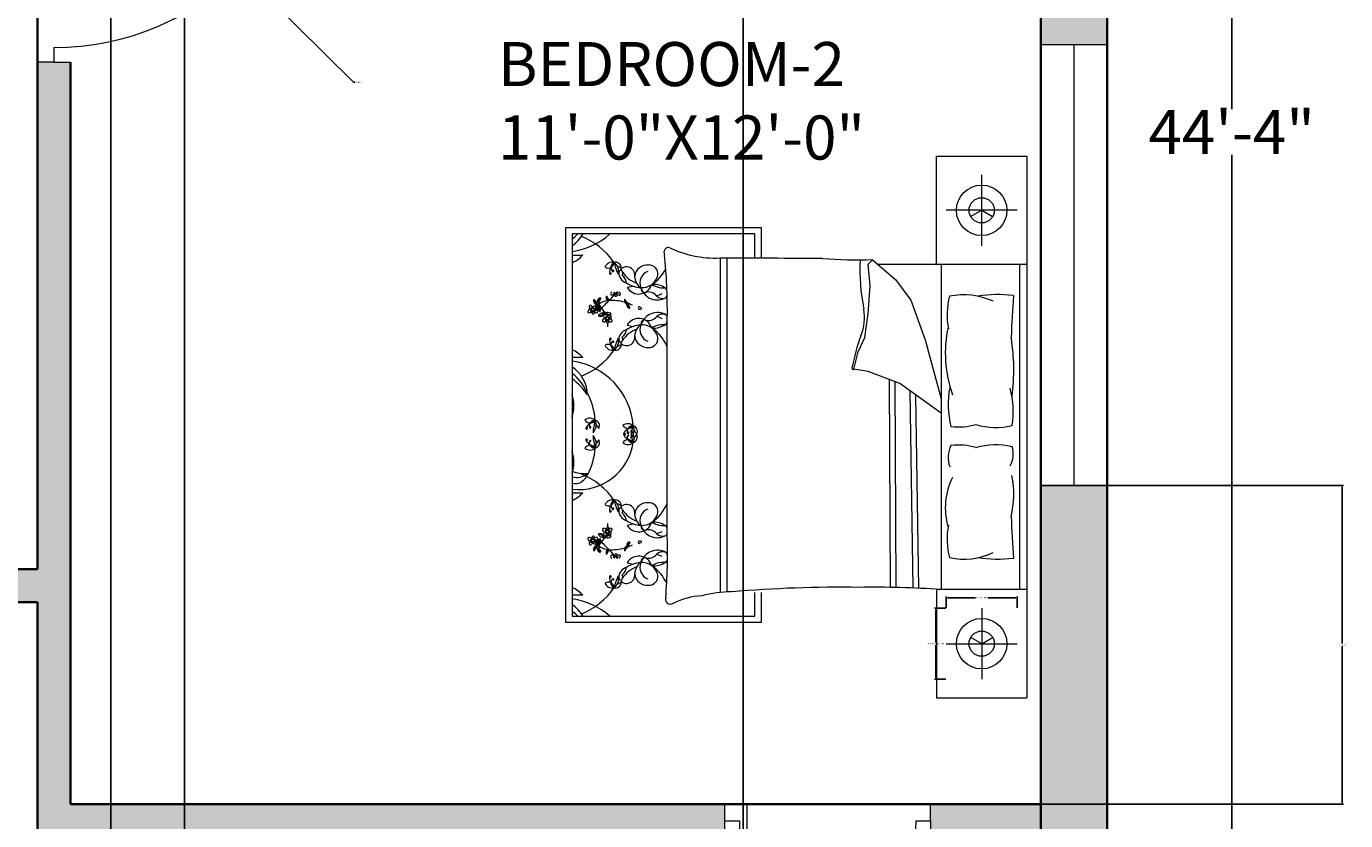
# Model space of a CAD drawing. Units: inches. Extents: x -13 to 349, y -556 to 61.
# Tile 3 of 6: x 170 to 349, y -351 to -243. Entities that reach past the tile are written whole.
import ezdxf

# ---------------------------------------------------------------- set-up
doc = ezdxf.new("R2010")
doc.units = ezdxf.units.IN
doc.header["$MEASUREMENT"] = 0
for name, color, linetype, lineweight in [('A-ANNO-DIMS', 2, 'Continuous', 18), ('A-AREA-IDEN', 7, 'Continuous', 18), ('A-DOOR', 3, 'Continuous', 20), ('A-FURN', 8, 'Continuous', 13), ('A-GLAZ', 5, 'Continuous', 18), ('A-WALL', 7, 'Continuous', 35), ('A-WALL-PATT', 8, 'Continuous', 13)]:
    doc.layers.add(name, color=color, linetype=linetype, lineweight=lineweight)
doc.styles.get("Standard").update_dxf_attribs({"font": 'arial.ttf'})
doc.dimstyles.get("Standard").update_dxf_attribs({"dimtxt": 0.18, "dimasz": 0.18, "dimexe": 0.18, "dimexo": 0.0625, "dimgap": 0.09, "dimtad": 0, "dimtih": 1, "dimtoh": 1, "dimdec": 0, "dimzin": 0, "dimdsep": 46, "dimlunit": 3, "dimtxsty": 'Standard', "dimcen": 0.09, "dimadec": 0, "dimazin": 0, "dimtfac": 1, "dimtdec": 0, "dimtofl": 0, "dimtmove": 0, "dimatfit": 3, "dimfxl": 1, "dimtolj": 1, "dimtzin": 0, "dimarcsym": 0})

# ---------------------------------------------------------------- blocks, each defined once
blk = doc.blocks.new('*D3')
at = {"layer": 'A-ANNO-DIMS', "color": 0, "lineweight": -2, "transparency": 16777216}
for p, q in [((316.82, 8.29), (333.9, 8.29)), ((333.72, 8.11), (333.72, -254.62)), ((333.72, -523.53), (333.72, -260.8)), ((316.82, -523.71), (333.9, -523.71))]:
    blk.add_line(p, q, dxfattribs=at)
at = {"layer": 'A-ANNO-DIMS', "color": 0, "transparency": 16777216}
for points in [[(333.69, 8.11), (333.75, 8.11), (333.72, 8.29)], [(333.69, -523.53), (333.75, -523.53), (333.72, -523.71)]]:
    blk.add_solid(points, dxfattribs=at)
at = {"layer": 'Defpoints', "color": 0, "transparency": 16777216}
for p in [(316.76, 8.29), (316.76, -523.71), (333.72, -523.71)]:
    blk.add_point(p, dxfattribs=at)
at = {"layer": 'A-ANNO-DIMS', "color": 0, "transparency": 16777216, "insert": (333.72, -257.71), "char_height": 6, "attachment_point": 5}
blk.add_mtext('\\A1;44\'-4"', dxfattribs=at)
blk = doc.blocks.new('DOOR-SWING-36IN')
for p, q in [((36, 40), (33.75, 40)), ((36, 38), (36, 40)), ((36, 40), (38.25, 40)), ((38.25, 3), (0, 3)), ((36, 2), (0, 2)), ((36, 0), (36, 2)), ((33.75, 0), (38.25, 0))]:
    blk.add_line(p, q)
blk.add_arc((36, 2), 36, 90, 180)
blk = doc.blocks.new('DOOR-SWING-24IN')
for p, q in [((4.5, 28), (0, 28)), ((2.25, 28), (2.25, 26)), ((2.25, 26), (26.25, 26)), ((0, 25), (26.25, 25)), ((2.25, 2), (2.25, 0)), ((2.25, 0), (0, 0)), ((2.25, 0), (4.5, 0))]:
    blk.add_line(p, q)
blk.add_arc((2.25, 26), 24, 270, 0)
blk = doc.blocks.new('WIN-60IN-D9')
for p, q in [((0, 60), (0, 0)), ((9, 60), (0, 60)), ((4.5, 60), (4.5, 0)), ((9, 0), (9, 60)), ((0, 0), (9, 0))]:
    blk.add_line(p, q)
blk = doc.blocks.new('BEDSIDE-LAMP-SM')
for p, q in [((4.82, 9.64), (4.82, 0)), ((0, 4.82), (9.64, 4.82))]:
    blk.add_line(p, q)
for points in [[(4.82, 4.82), (3.33, 5.68)], [(4.82, 4.82), (6.31, 5.68)]]:
    blk.add_lwpolyline(points)
for radius in [3.44, 1.72]:
    blk.add_circle((4.82, 4.82), radius)
blk = doc.blocks.new('*D32')
at = {"layer": 'A-ANNO-DIMS', "color": 0, "lineweight": -2, "transparency": 16777216}
for p, q in [((294.83, -322.55), (293.27, -322.55)), ((293.45, -322.73), (293.45, -327.19)), ((293.45, -332.01), (293.45, -327.55)), ((294.83, -332.19), (293.27, -332.19))]:
    blk.add_line(p, q, dxfattribs=at)
at = {"layer": 'A-ANNO-DIMS', "color": 0, "transparency": 16777216}
for points in [[(293.42, -322.73), (293.48, -322.73), (293.45, -322.55)], [(293.42, -332.01), (293.48, -332.01), (293.45, -332.19)]]:
    blk.add_solid(points, dxfattribs=at)
at = {"layer": 'Defpoints', "color": 0, "transparency": 16777216}
for p in [(293.45, -322.55), (294.89, -322.55), (294.89, -332.19)]:
    blk.add_point(p, dxfattribs=at)
at = {"layer": 'A-ANNO-DIMS', "color": 0, "transparency": 16777216, "insert": (293.45, -327.37), "char_height": 0.18, "attachment_point": 5}
blk.add_mtext('\\A1;LAMP B 0\'-9 1/2" TYP.', dxfattribs=at)
blk = doc.blocks.new('*D33')
at = {"layer": 'A-ANNO-DIMS', "color": 0, "lineweight": -2, "transparency": 16777216}
for p, q in [((294.89, -322.49), (294.89, -320.93)), ((295.07, -321.11), (298.86, -321.11)), ((304.35, -321.11), (300.56, -321.11)), ((304.53, -322.49), (304.53, -320.93))]:
    blk.add_line(p, q, dxfattribs=at)
at = {"layer": 'A-ANNO-DIMS', "color": 0, "transparency": 16777216}
for points in [[(295.07, -321.08), (295.07, -321.14), (294.89, -321.11)], [(304.35, -321.08), (304.35, -321.14), (304.53, -321.11)]]:
    blk.add_solid(points, dxfattribs=at)
at = {"layer": 'Defpoints', "color": 0, "transparency": 16777216}
for p in [(304.53, -321.11), (294.89, -322.55), (304.53, -322.55)]:
    blk.add_point(p, dxfattribs=at)
at = {"layer": 'A-ANNO-DIMS', "color": 0, "transparency": 16777216, "insert": (299.71, -321.11), "char_height": 0.18, "attachment_point": 5}
blk.add_mtext('\\A1;0\'-9 1/2" TYP.', dxfattribs=at)
blk = doc.blocks.new('*D34')
at = {"layer": 'A-ANNO-DIMS', "color": 0, "lineweight": -2, "transparency": 16777216}
for p, q in [((267.26, -200.78), (267.26, -555.89)), ((307.76, -200.78), (307.76, -555.89)), ((267.44, -555.71), (286.97, -555.71)), ((307.58, -555.71), (288.04, -555.71))]:
    blk.add_line(p, q, dxfattribs=at)
at = {"layer": 'A-ANNO-DIMS', "color": 0, "transparency": 16777216}
for points in [[(267.44, -555.68), (267.44, -555.74), (267.26, -555.71)], [(307.58, -555.68), (307.58, -555.74), (307.76, -555.71)]]:
    blk.add_solid(points, dxfattribs=at)
at = {"layer": 'Defpoints', "color": 0, "transparency": 16777216}
for p in [(267.26, -200.71), (307.76, -200.71), (307.76, -555.71)]:
    blk.add_point(p, dxfattribs=at)
at = {"layer": 'A-ANNO-DIMS', "color": 0, "transparency": 16777216, "insert": (287.51, -555.71), "char_height": 0.18, "attachment_point": 5}
blk.add_mtext('\\A1;3\'-4 1/2"', dxfattribs=at)
blk = doc.blocks.new('*D37')
at = {"layer": 'A-ANNO-DIMS', "color": 0, "lineweight": -2, "transparency": 16777216}
for p, q in [((181.26, -353.65), (181.26, 40.47)), ((181.44, 40.29), (185.86, 40.29)), ((191.08, 40.29), (186.65, 40.29)), ((191.26, -353.65), (191.26, 40.47))]:
    blk.add_line(p, q, dxfattribs=at)
at = {"layer": 'A-ANNO-DIMS', "color": 0, "transparency": 16777216}
for points in [[(181.44, 40.32), (181.44, 40.26), (181.26, 40.29)], [(191.08, 40.32), (191.08, 40.26), (191.26, 40.29)]]:
    blk.add_solid(points, dxfattribs=at)
at = {"layer": 'Defpoints', "color": 0, "transparency": 16777216}
for p in [(191.26, 40.29), (181.26, -353.71), (191.26, -353.71)]:
    blk.add_point(p, dxfattribs=at)
at = {"layer": 'A-ANNO-DIMS', "color": 0, "transparency": 16777216, "insert": (186.26, 40.29), "char_height": 0.18, "attachment_point": 5}
blk.add_mtext('\\A1;0\'-10"', dxfattribs=at)
blk = doc.blocks.new('*D42')
at = {"layer": 'A-ANNO-DIMS', "color": 0, "lineweight": -2, "transparency": 16777216}
for p, q in [((307.82, -305.84), (348.94, -305.84)), ((348.76, -306.02), (348.76, -327.34)), ((348.76, -349.03), (348.76, -327.71)), ((307.82, -349.21), (348.94, -349.21))]:
    blk.add_line(p, q, dxfattribs=at)
at = {"layer": 'A-ANNO-DIMS', "color": 0, "transparency": 16777216}
for points in [[(348.73, -306.02), (348.79, -306.02), (348.76, -305.84)], [(348.73, -349.03), (348.79, -349.03), (348.76, -349.21)]]:
    blk.add_solid(points, dxfattribs=at)
at = {"layer": 'Defpoints', "color": 0, "transparency": 16777216}
for p in [(307.76, -305.84), (307.76, -349.21), (348.76, -349.21)]:
    blk.add_point(p, dxfattribs=at)
at = {"layer": 'A-ANNO-DIMS', "color": 0, "transparency": 16777216, "insert": (348.76, -327.53), "char_height": 0.18, "attachment_point": 5}
blk.add_mtext('\\A1;3\'-7 1/2"', dxfattribs=at)
blk = doc.blocks.new('*D48')
at = {"layer": 'A-ANNO-DIMS', "color": 0, "lineweight": -2, "transparency": 16777216}
for p, q in [((173.42, -210.21), (173.6, -210.21)), ((173.51, -210.3), (173.51, -210.12)), ((214.24, -250.94), (199.09, -235.8)), ((214.42, -250.94), (214.24, -250.94))]:
    blk.add_line(p, q, dxfattribs=at)
at = {"layer": 'A-ANNO-DIMS', "color": 0, "transparency": 16777216}
blk.add_solid([(199.11, -235.77), (199.07, -235.82), (198.96, -235.67)], dxfattribs=at)
at = {"layer": 'Defpoints', "color": 0, "transparency": 16777216}
for p in [(173.51, -210.21), (198.96, -235.67)]:
    blk.add_point(p, dxfattribs=at)
at = {"layer": 'A-ANNO-DIMS', "color": 0, "transparency": 16777216, "insert": (215.03, -250.94), "char_height": 0.18, "attachment_point": 5}
blk.add_mtext('\\A1;4X R3\'-0"', dxfattribs=at)

msp = doc.modelspace()

# ---------------------------------------------------------------- hatches: boundary and pattern name
at = {"layer": 'A-WALL-PATT'}
h = msp.add_hatch(color=256, dxfattribs=at)
h.dxf.hatch_style = 1
h.paths.add_polyline_path([(316.76, 8.29), (171.26, 8.29), (171.26, -0.71), (307.76, -0.71), (307.76, -52.19), (316.76, -52.19)])
h.paths.add_polyline_path([(175.76, -0.71), (171.26, -0.71), (171.26, -82.21), (165.24, -82.21), (165.24, -86.71), (171.26, -86.71), (171.26, -101.71), (173.51, -101.71), (175.76, -101.71)])
h.paths.add_polyline_path([(171.26, -25.21), (165.17, -25.21), (165.17, -34.21), (171.26, -34.21)])
h.paths.add_polyline_path([(141.17, -25.21), (127.76, -25.21), (127.76, -34.21), (141.17, -34.21)])
h.paths.add_polyline_path([(28.76, -25.21), (24.26, -25.21), (19.76, -25.21), (19.76, -78.88), (28.76, -78.88)])
h.paths.add_polyline_path([(99.76, -29.71), (99.76, -25.21), (28.76, -25.21), (28.76, -34.21), (99.76, -34.21)])
h.paths.add_polyline_path([(135.26, -86.71), (143.68, -86.71), (143.68, -82.21), (135.26, -82.21), (135.26, -34.21), (130.76, -34.21), (130.76, -101.71), (133.01, -101.71), (135.26, -101.71)])
h.paths.add_polyline_path([(135.26, -141.71), (130.76, -141.71), (130.76, -144.71), (28.76, -144.71), (28.76, -149.21), (135.26, -149.21)])
h.paths.add_polyline_path([(28.76, -138.88), (19.76, -138.88), (19.76, -156.62), (28.76, -156.62)])
h.paths.add_polyline_path([(28.76, -192.62), (19.76, -192.62), (19.76, -271.06), (28.76, -271.06)])
h.paths.add_polyline_path([(28.76, -307.06), (19.76, -307.06), (19.76, -385.56), (28.76, -385.56)])
h.paths.add_polyline_path([(28.76, -445.56), (19.76, -445.56), (19.76, -523.71), (28.76, -523.71)])
h.paths.add_polyline_path([(307.76, -431.71), (261.76, -431.71), (261.76, -353.71), (264.76, -353.71), (264.76, -349.21), (175.76, -349.21), (175.76, -248.21), (173.51, -248.21), (171.26, -248.21), (171.26, -317.21), (168.26, -317.21), (168.26, -321.71), (171.26, -321.71), (171.26, -353.71), (257.26, -353.71), (257.26, -431.71), (171.26, -431.71), (171.26, -436.21), (307.76, -436.21)])
h.paths.add_polyline_path([(316.76, -424.85), (307.76, -424.85), (307.76, -436.21), (316.76, -436.21)])
h.paths.add_polyline_path([(316.76, -305.84), (307.76, -305.84), (307.76, -400.85), (316.76, -400.85)])
h.paths.add_polyline_path([(307.76, -349.21), (292.76, -349.21), (292.76, -351.46), (292.76, -353.71), (307.76, -353.71)], flags=17)
h.paths.add_polyline_path([(271.19, -200.71), (267.26, -200.71), (267.26, -186.96), (262.76, -186.96), (262.76, -200.71), (175.76, -200.71), (175.76, -180.21), (173.51, -180.21), (171.26, -180.21), (171.26, -208.21), (175.76, -208.21), (175.76, -205.21), (271.19, -205.21)])
h.paths.add_polyline_path([(316.76, -112.19), (307.76, -112.19), (307.76, -245.84), (316.76, -245.84)])
h.paths.add_polyline_path([(271.33, -144.71), (175.76, -144.71), (175.76, -141.71), (171.26, -141.71), (171.26, -152.21), (175.76, -152.21), (175.76, -149.21), (262.76, -149.21), (262.76, -162.96), (267.26, -162.96), (267.26, -149.21), (271.33, -149.21)])
h.paths.add_polyline_path([(307.76, -200.71), (307.19, -200.71), (307.19, -205.21), (307.76, -205.21)])
h.paths.add_polyline_path([(307.76, -144.71), (307.33, -144.71), (307.33, -149.21), (307.76, -149.21)])

# ---------------------------------------------------------------- linework, layer by layer
at = {"layer": 'A-FURN'}
for p, q in [((305.85, -261), (305.85, -334.74)), ((243.14, -270.73), (269.7, -270.73)), ((243.14, -324.5), (243.14, -270.73)), ((269.7, -270.73), (269.7, -274.9)), ((243.99, -271.59), (243.99, -323.64)), ((268.85, -271.59), (243.99, -271.59)), ((268.85, -274.9), (268.85, -271.59)), ((264.19, -320.4), (264.19, -274.9)), ((265.1, -320.33), (265.1, -274.9)), ((284.25, -275.68), (284.84, -275.09)), ((284.55, -278.67), (284.25, -275.68)), ((284.84, -275.09), (287.98, -277.78)), ((305.85, -275.75), (285.61, -275.75)), ((294.2, -275.75), (294.2, -320)), ((304.91, -320), (304.91, -275.75)), ((287.98, -277.78), (290.07, -280.61)), ((251.47, -278.85), (252.3, -278.69)), ((284.25, -282.41), (284.55, -278.67)), ((290.07, -280.61), (292.01, -285.99)), ((256.94, -312.84), (256.94, -282.9)), ((283.8, -285.69), (284.25, -282.41)), ((251.47, -284.01), (252.3, -284.17)), ((282.9, -287.63), (283.8, -285.69)), ((292.01, -285.99), (294.2, -294.03)), ((282.31, -290.02), (282.9, -287.63)), ((284.25, -290.32), (282.31, -290.02)), ((288.58, -291.97), (284.25, -290.32)), ((287.3, -319.73), (287.19, -291.44)), ((288.06, -319.73), (287.95, -291.73)), ((294.2, -296.01), (288.58, -291.97)), ((290.38, -319.77), (290, -292.99)), ((291.14, -319.8), (290.77, -293.54)), ((251.47, -311.22), (252.3, -311.06)), ((251.47, -316.37), (252.3, -316.54)), ((268.85, -323.64), (268.85, -320.39)), ((269.7, -320.41), (269.7, -324.5)), ((269.7, -324.5), (243.14, -324.5)), ((243.99, -323.64), (268.85, -323.64))]:
    msp.add_line(p, q, dxfattribs=at)
for points in [[(293.56, -275.75), (293.56, -261), (305.85, -261)], [(305.85, -320), (293.56, -320), (293.56, -334.74), (305.85, -334.74)]]:
    msp.add_lwpolyline(points, dxfattribs=at)
for points in [[(278.09, -274.93, 0.001242), (264.1, -274.9, -0.127202), (257.13, -273.42)], [(304.02, -279.98, 0.074897), (299.2, -280.07, -0.472817)], [(298.93, -297.53, 0.14099), (303.84, -297.67, 0.235245)], [(298.93, -300.67, -0.14099), (303.84, -300.53, -0.235245)], [(304.02, -315.76, -0.074897), (299.2, -315.67, 0.472817)], [(265.69, -320.31, 0.056112), (261.63, -320.84, 0.095341), (257.72, -321.88)]]:
    msp.add_lwpolyline(points, format="xyb", dxfattribs=at)
for centre in [(246.82, -281.89), (248.8, -283.11), (248.8, -312.11), (246.82, -313.34)]:
    msp.add_circle(centre, 0.188, dxfattribs=at)
for centre, radius, start, end in [((240.53, -267.56), 5.85, 306.3036, 316.4814), ((241.41, -269.25), 4.69, 303.4617, 330.1116), ((242.7, -264.42), 9.63, 277.745, 311.8856), ((241.74, -280.89), 9.63, 34.3865, 68.5908), ((242.49, -271.88), 3.92, 292.5547, 318.9546), ((244.6, -261.15), 13.32, 267.4081, 273.6519), ((257.17, -274.1), 0.68, 93.98, 207.3412), ((180.18, -282.02), 76.77, 359.3433, 5.6887), ((249.46, -276.5), 1.07, 77.7115, 159.0387), ((248.89, -275.43), 0.804, 238.4633, 358.2869), ((251.52, -277.06), 2.44, 138.8402, 177.9352), ((250.06, -276.15), 0.788, 117.6827, 223.7762), ((249.88, -276.23), 0.798, 2.9516, 103.728), ((256.27, -273.99), 6.74, 192.5173, 207.1824), ((248.8, -276.69), 1.52, 345.4653, 54.2343), ((251.1, -274.6), 1.64, 211.3827, 255.2969), ((251.41, -277.17), 1.11, 350.264, 160.8688), ((254.25, -277.57), 1.76, 84.9449, 172.8857), ((254.43, -277.06), 1.25, 354.4856, 91.0538), ((251.75, -273.81), 5.58, 303.6671, 333.2997), ((283.01, -207.47), 67.64, 265.8294, 271.553), ((310.96, -276.35), 27.83, 177.4519, 191.3392), ((249.21, -276.97), 0.12, 177.9352, 11.4834), ((249.27, -276.96), 0.0581, 11.4834, 127.9409), ((249.56, -276.62), 0.104, 223.7762, 159.7183), ((251.74, -276.9), 1.38, 175.969, 254.3045), ((250.21, -276.94), 0.678, 333.9755, 53.2681), ((249.91, -278.39), 1.47, 6.1662, 51.5825), ((253.85, -274.97), 3.48, 211.2614, 251.7045), ((254.64, -277.27), 2.14, 182.3591, 234.0401), ((254.92, -278.27), 1.71, 111.5819, 201.4221), ((253.51, -276.68), 2.22, 265.2933, 346.921), ((244.23, -275.55), 7, 313.1541, 322.0459), ((249.38, -279.76), 0.144, 142.4737, 265.053), ((249.57, -279.73), 0.31, 127.7621, 169.0403), ((249.4, -279.47), 0.436, 265.053, 338.3618), ((249.98, -280.06), 0.57, 113.4276, 137.6104), ((249.91, -279.47), 0.188, 183.2768, 356.7232), ((250.05, -279.81), 0.307, 139.7889, 227.6792), ((249.95, -279.92), 0.162, 227.6792, 350.3487), ((249.33, -279.81), 0.615, 353.0852, 15.7171), ((249.73, -279.88), 0.388, 350.3487, 43.6538), ((250.45, -279.48), 0.452, 198.7263, 262.5032), ((250.09, -279.69), 0.179, 1.1081, 91.8675), ((250.2, -279.73), 0.313, 11.5637, 52.6358), ((250.43, -279.79), 0.145, 255.2356, 54.9248), ((253.57, -274.94), 3.96, 236.2883, 266.5076), ((253.06, -277.94), 1.83, 209.9085, 343.1337), ((253.83, -279.1), 0.458, 167.3041, 285.1471), ((255.07, -281.29), 2.84, 122.7011, 126.3445), ((255.6, -278.22), 2.35, 199.2822, 299.1751), ((254.34, -281), 1.51, 41.5653, 105.1471), ((256.4, -275.86), 3.06, 238.8218, 279.1554), ((255.07, -281.29), 2.84, 55.785, 94.7304), ((255.18, -277.87), 2.12, 277.436, 299.9149), ((256.13, -279.64), 0.888, 30.0293, 52.325), ((297.27, -289.38), 9.5, 65.1316, 101.7583), ((246.67, -281.5), 0.371, 157.4086, 261.4386), ((246.47, -281.49), 0.186, 58.0499, 135.6268), ((246.66, -281.61), 0.124, 172.906, 277.132), ((246.25, -281.84), 0.592, 14.7558, 58.0499), ((247.08, -281.68), 0.256, 36.1046, 181.4281), ((247.09, -280.67), 0.21, 124.3538, 214.3923), ((247.4, -280.71), 0.489, 190.3057, 287.1958), ((246.93, -281.48), 0.259, 270.0645, 331.1507), ((247.15, -281.54), 0.295, 221.8413, 265.7877), ((247.54, -280.53), 0.568, 176.9701, 248.2913), ((251.59, -277.54), 5.49, 212.6784, 216.3746), ((247.15, -281.65), 0.184, 263.7526, 41.7054), ((247.35, -280.66), 0.217, 216.3746, 291.7548), ((249.27, -283.71), 3.06, 124.0033, 132.4917), ((246.12, -284.1), 3.27, 63.7819, 68.2913), ((247.87, -281.58), 0.52, 128.3208, 208.8162), ((247.87, -280.82), 0.489, 122.8155, 187.3992), ((247.49, -281.02), 0.164, 289.3605, 111.7548), ((247.61, -281.02), 0.164, 221.8703, 44.2646), ((248.36, -281.49), 0.856, 157.2305, 229.0635), ((248.08, -280.88), 0.568, 109.4799, 177.6828), ((248.07, -281.21), 0.504, 174.4544, 220.6188), ((245.2, -284.03), 3.67, 30.544, 49.818), ((247.78, -280.52), 0.21, 56.8636, 146.9021), ((247.89, -280.75), 0.217, 148.8844, 224.2646), ((247.23, -281.93), 0.606, 340.0041, 40.6188), ((252.4, -283.48), 5.49, 145.1882, 148.8844), ((249.27, -283.71), 3.06, 94.756, 119.2041), ((255.79, -288.12), 10.08, 132.2412, 142.1744), ((250.7, -280.1), 2.08, 178.3264, 187.1302), ((248.46, -280.39), 0.387, 11.3256, 64.4621), ((249.77, -279.83), 1.17, 190.2588, 210.656), ((248.99, -280.31), 0.354, 188.3432, 274.2869), ((249.3, -280.11), 0.618, 210.656, 242.6341), ((249.77, -279.58), 1.18, 218.2101, 226.3071), ((248.89, -280.58), 0.15, 325.7657, 67.4417), ((249.42, -286.75), 6.11, 73.5842, 93.8277), ((253.18, -280.54), 2.08, 178.3264, 187.1302), ((250.94, -280.83), 0.387, 11.3256, 64.4621), ((252.25, -280.27), 1.17, 190.2588, 210.656), ((251.47, -280.75), 0.354, 188.3432, 274.2869), ((251.78, -280.55), 0.618, 210.656, 242.6341), ((252.25, -280.02), 1.18, 218.2101, 226.3071), ((251.37, -281.01), 0.15, 325.7657, 67.4417), ((251.8, -281.29), 0.354, 147.5332, 233.4768), ((252.12, -281.11), 0.618, 179.1859, 211.164), ((251.51, -281.25), 0.15, 354.3784, 96.0543), ((249.42, -286.75), 6.11, 63.0032, 69.8941), ((252.58, -280.82), 1.17, 211.164, 231.5612), ((252.79, -279.88), 2.08, 234.6898, 243.4936), ((252.8, -280.95), 1.18, 195.5129, 203.6099), ((251.47, -281.72), 0.387, 357.3579, 50.4944), ((253.14, -281.64), 0.142, 12.7051, 190.4384), ((253.22, -281.63), 0.231, 190.4384, 10.4136), ((256.3, -279.27), 1.1, 221.5653, 293.8354), ((256.13, -279.64), 0.888, 314.4517, 333.558), ((304.88, -282.61), 9.88, 165.1039, 191.0369), ((1005.83, -320.63), 702.99, 176.68521, 177.14978), ((246.28, -282.17), 0.144, 142.4737, 265.053), ((246.47, -282.14), 0.31, 61.2196, 169.0403), ((246.31, -281.88), 0.436, 265.053, 338.3618), ((246.88, -282.48), 0.57, 113.4276, 137.6104), ((246.96, -282.23), 0.307, 139.7889, 227.6792), ((246.86, -282.33), 0.162, 227.6792, 350.3487), ((246.23, -282.22), 0.615, 353.0852, 15.7171), ((246.64, -282.3), 0.388, 350.3487, 43.6538), ((247.35, -281.89), 0.452, 198.7263, 262.5032), ((247, -282.1), 0.179, 1.1081, 91.8675), ((247.11, -282.15), 0.313, 11.5637, 86.365), ((247.33, -282.2), 0.145, 255.2356, 54.9248), ((247.96, -281.54), 0.622, 207.7043, 254.3516), ((247.56, -281.9), 0.856, 270.278, 342.111), ((248.13, -282.97), 0.606, 98.7227, 159.3375), ((247.82, -282.19), 0.622, 244.9899, 291.6373), ((247.96, -281.87), 0.504, 278.7227, 324.8872), ((247.87, -282.28), 0.52, 290.5253, 358.5375), ((248.26, -283.4), 0.144, 142.4737, 265.053), ((248.45, -283.37), 0.31, 61.2196, 169.0403), ((248.29, -283.11), 0.436, 265.053, 338.3618), ((248.65, -282.73), 0.371, 157.4086, 261.4386), ((248.45, -282.72), 0.186, 58.0499, 135.6268), ((248.89, -282.13), 0.52, 182.8499, 266.1226), ((248.68, -281.77), 0.504, 231.7607, 277.9252), ((249.08, -281.68), 0.856, 214.5369, 286.3699), ((248.86, -283.7), 0.57, 113.4276, 137.6104), ((248.64, -282.84), 0.124, 172.906, 277.132), ((248.23, -283.06), 0.592, 14.7558, 58.0499), ((245.2, -284.03), 3.67, 23.0501, 23.8477), ((248.94, -283.45), 0.307, 139.7889, 227.6792), ((248.84, -282.87), 0.606, 37.3105, 97.9252), ((249.06, -282.91), 0.256, 36.1046, 181.4281), ((248.21, -283.45), 0.615, 353.0852, 15.7171), ((248.9, -282.03), 0.622, 265.0106, 311.658), ((248.61, -283.52), 0.388, 350.3487, 43.6538), ((248.91, -282.71), 0.259, 270.0645, 331.1507), ((249.13, -282.77), 0.295, 221.8413, 265.7877), ((249.33, -283.12), 0.452, 198.7263, 262.5032), ((248.98, -283.33), 0.179, 1.1081, 91.8675), ((249.13, -282.88), 0.184, 263.7526, 41.7054), ((249.09, -283.37), 0.313, 11.5637, 86.365), ((249.31, -283.43), 0.145, 255.2356, 54.9248), ((253.06, -284.92), 1.83, 16.8663, 150.0915), ((253.83, -283.76), 0.458, 74.8529, 192.6959), ((255.6, -284.64), 2.35, 60.8249, 160.7178), ((254.34, -281.86), 1.51, 254.8529, 318.4347), ((255.18, -284.99), 2.12, 60.0851, 82.564), ((256.3, -283.6), 1.1, 66.1646, 138.4347), ((256.13, -283.22), 0.888, 23.229, 45.5483), ((277.78, -283), 6, 336.2616, 11.3392), ((248.84, -283.56), 0.162, 227.6792, 350.3487), ((245.2, -284.03), 3.67, 357.1071, 4.7585), ((251.74, -285.96), 1.38, 105.6955, 184.031), ((249.91, -284.47), 1.47, 308.4175, 353.8338), ((253.85, -287.89), 3.48, 108.2955, 148.7386), ((253.57, -287.92), 3.96, 93.4924, 123.7117), ((254.64, -285.6), 2.14, 125.9599, 177.6409), ((254.92, -284.6), 1.71, 158.5779, 248.4181), ((253.51, -286.18), 2.22, 13.079, 94.7067), ((255.07, -281.57), 2.84, 233.6555, 237.2989), ((256.4, -287), 3.06, 79.7133, 121.1782), ((255.07, -281.57), 2.84, 265.2696, 304.215), ((251.75, -289.05), 5.58, 21.4941, 56.3329), ((256.13, -283.22), 0.888, 307.675, 336.7144), ((311.9, -287.82), 17.14, 168.0397, 199.2615), ((248.89, -287.43), 0.804, 1.7131, 121.5367), ((249.46, -286.36), 1.07, 200.9613, 282.2885), ((249.21, -285.89), 0.12, 348.5166, 182.0648), ((251.52, -285.8), 2.44, 182.0648, 221.1598), ((249.27, -285.9), 0.0581, 232.0591, 348.5166), ((250.06, -286.71), 0.788, 136.2238, 242.3173), ((249.6, -286.25), 0.0628, 200.2667, 136.2271), ((248.8, -286.17), 1.52, 305.7657, 14.5347), ((256.27, -288.87), 6.74, 152.8176, 167.4827), ((249.88, -286.63), 0.798, 256.272, 357.0484), ((251.1, -288.26), 1.64, 104.7031, 148.6173), ((251.41, -285.69), 1.11, 199.1312, 9.736), ((250.21, -285.92), 0.678, 306.7319, 26.0245), ((254.25, -285.29), 1.76, 187.1143, 275.0551), ((254.43, -285.8), 1.25, 268.9462, 5.5144), ((310.17, -295.14), 28.6, 160.1194, 169.3383), ((277.33, -290.09), 26.75, 352.2196, 9.497), ((242.49, -290.99), 3.92, 41.0454, 67.4453), ((244.6, -301.71), 13.32, 86.3481, 92.5919), ((242.7, -298.44), 9.63, 4.4623, 82.255), ((241.74, -281.97), 9.63, 291.4092, 325.6135), ((241.41, -293.61), 4.69, 1.272, 56.5383), ((240.53, -295.3), 5.85, 17.8504, 53.6964), ((282.25, -289.86), 0.178, 178.8623, 289.7536), ((238.89, -298.37), 8.7, 34.0123, 54.053), ((308.16, -294.76), 13, 169.8617, 193.6238), ((238.93, -295.01), 5.3, 343.5431, 17.0202), ((237.54, -297.71), 9.63, 4.4623, 27.4146), ((290.85, -295.74), 13.14, 351.5249, 13.96), ((236.2, -297.11), 7.83, 4.3787, 5.6357), ((230.84, -301.24), 13.99, 19.7217, 19.9028), ((246.42, -297.75), 1.07, 47.7873, 129.1145), ((246.45, -296.54), 0.804, 208.5391, 328.3627), ((247.93, -299.26), 2.44, 108.9159, 148.011), ((247.11, -297.75), 0.788, 87.7585, 193.852), ((246.44, -297.91), 0.104, 193.852, 129.9245), ((253.57, -298.97), 6.74, 162.593, 177.2582), ((245.75, -297.58), 1.52, 315.5411, 24.3101), ((248.78, -296.92), 1.64, 181.4585, 225.3727), ((246.92, -297.72), 0.798, 333.0274, 73.8037), ((251.58, -298.49), 1.07, 47.7873, 129.1145), ((251.61, -297.27), 0.804, 208.5391, 328.3627), ((253.09, -300), 2.44, 108.9159, 148.011), ((252.27, -298.48), 0.788, 87.7585, 193.852), ((250.91, -298.32), 1.52, 315.5411, 24.3101), ((258.73, -299.71), 6.74, 162.593, 177.2582), ((252.07, -298.46), 0.798, 333.0274, 73.8037), ((253.94, -297.65), 1.64, 181.4585, 225.3727), ((296.47, -288.83), 9.04, 264.0129, 285.8293), ((245.96, -298.04), 0.12, 148.011, 341.5592), ((245.96, -299.65), 0.12, 18.4408, 211.989), ((246.02, -298.05), 0.0581, 341.5592, 98.0167), ((246.02, -299.63), 0.0581, 261.9833, 18.4408), ((253.57, -298.71), 6.74, 182.7418, 197.407), ((245.75, -300.1), 1.52, 335.6899, 44.4589), ((248.78, -300.77), 1.64, 134.6273, 178.5415), ((246.92, -299.96), 0.798, 286.1963, 26.9726), ((251.61, -300.41), 0.804, 31.6373, 151.4609), ((251.12, -298.77), 0.12, 148.011, 341.5592), ((251.12, -298.91), 0.12, 18.4408, 211.989), ((253.09, -297.69), 2.44, 211.989, 251.0841), ((251.18, -298.79), 0.0581, 341.5592, 98.0167), ((251.18, -298.89), 0.0581, 261.9833, 18.4408), ((252.27, -299.2), 0.788, 166.148, 272.2415), ((251.6, -298.65), 0.104, 193.852, 129.9245), ((251.64, -299.03), 0.0628, 230.1909, 166.0209), ((250.91, -299.36), 1.52, 335.6899, 44.4589), ((258.73, -297.98), 6.74, 182.7418, 197.407), ((252.07, -299.22), 0.798, 286.1963, 26.9726), ((253.94, -300.03), 1.64, 134.6273, 178.5415), ((244.92, -298.93), 7.45, 262.8636, 351.8197), ((238.93, -302.67), 5.3, 342.9798, 16.4569), ((236.2, -300.57), 7.83, 354.3643, 355.6213), ((230.84, -296.45), 13.99, 340.0972, 340.2783), ((246.45, -301.15), 0.804, 31.6373, 151.4609), ((246.42, -299.94), 1.07, 230.8855, 312.2127), ((247.93, -298.42), 2.44, 211.989, 251.0841), ((237.54, -299.98), 9.63, 332.5854, 355.5377), ((247.11, -299.94), 0.788, 166.148, 272.2415), ((246.48, -299.77), 0.0628, 230.1909, 166.0209), ((251.58, -299.2), 1.07, 230.8855, 312.2127), ((299.07, -302.03), 3.91, 155.0183, 198.5407), ((296.47, -309.37), 9.04, 74.1707, 95.9871), ((300.34, -301.54), 3.65, 333.3437, 16.1026), ((245.6, -299.89), 4.31, 248.117, 276.6195), ((244.4, -303.85), 1.73, 256.3898, 349.0739), ((244.64, -302.55), 2.19, 252.8609, 311.9049), ((241.74, -313.26), 9.63, 34.3865, 68.5908), ((304.15, -308.86), 9.39, 153.8761, 196.1746), ((291.11, -307.01), 12.96, 346.3427, 11.1841), ((244.6, -293.52), 13.32, 267.4081, 273.6519), ((242.49, -304.24), 3.92, 292.5547, 318.9546), ((249.46, -308.86), 1.07, 77.7115, 159.0387), ((248.89, -307.8), 0.804, 238.4633, 358.2869), ((251.52, -309.42), 2.44, 138.8402, 177.9352), ((250.06, -308.52), 0.788, 117.6827, 223.7762), ((249.88, -308.6), 0.798, 2.9516, 103.728), ((251.1, -306.96), 1.64, 211.3827, 255.2969), ((248.8, -309.06), 1.52, 345.4653, 54.2343), ((256.27, -306.36), 6.74, 192.5173, 207.1824), ((251.41, -309.53), 1.11, 350.264, 160.8688), ((254.25, -309.94), 1.76, 84.9449, 172.8857), ((254.43, -309.43), 1.25, 354.4856, 91.0538), ((251.75, -306.18), 5.58, 303.6671, 338.5059), ((249.21, -309.34), 0.12, 177.9352, 11.4834), ((249.27, -309.33), 0.0581, 11.4834, 127.9409), ((249.56, -308.99), 0.104, 223.7762, 159.7183), ((251.74, -309.27), 1.38, 175.969, 254.3045), ((250.21, -309.31), 0.678, 333.9755, 53.2681), ((249.91, -310.76), 1.47, 6.1662, 51.5825), ((253.85, -307.34), 3.48, 211.2614, 251.7045), ((254.64, -309.63), 2.14, 182.3591, 234.0401), ((254.92, -310.63), 1.71, 111.5819, 201.4221), ((253.51, -309.05), 2.22, 265.2933, 346.921), ((1005.83, -275.11), 702.99, 182.85022, 183.31479), ((248.26, -311.83), 0.144, 94.947, 217.5263), ((248.45, -311.86), 0.31, 190.9597, 298.7804), ((248.29, -312.12), 0.436, 21.6382, 94.947), ((248.65, -312.5), 0.371, 98.5614, 202.5914), ((248.86, -311.52), 0.57, 222.3896, 246.5724), ((248.94, -311.77), 0.307, 132.3208, 220.2111), ((248.84, -311.67), 0.162, 9.6513, 132.3208), ((248.21, -311.78), 0.615, 344.2829, 6.9148), ((245.2, -311.2), 3.67, 355.2415, 2.8929), ((248.61, -311.7), 0.388, 316.3462, 9.6513), ((249.33, -312.11), 0.452, 97.4968, 161.2737), ((249.13, -312.46), 0.295, 94.2123, 138.1587), ((248.98, -311.89), 0.179, 268.1325, 358.8919), ((249.09, -311.85), 0.313, 273.635, 348.4363), ((249.13, -312.35), 0.184, 318.2946, 96.2474), ((249.31, -311.8), 0.145, 305.0752, 104.7644), ((253.57, -307.31), 3.96, 236.2883, 266.5076), ((253.06, -310.31), 1.83, 209.9085, 343.1337), ((253.83, -311.47), 0.458, 167.3041, 285.1471), ((255.07, -313.66), 2.84, 122.7011, 126.3445), ((255.6, -310.59), 2.35, 199.2822, 299.1751), ((254.34, -313.37), 1.51, 41.5653, 105.1471), ((256.4, -308.22), 3.06, 238.8218, 280.2867), ((255.07, -313.66), 2.84, 55.785, 94.7304), ((255.18, -310.24), 2.12, 277.436, 299.9149), ((256.13, -312.01), 0.888, 23.2856, 52.325), ((304.88, -313.13), 9.88, 168.9631, 194.8961), ((246.28, -313.06), 0.144, 94.947, 217.5263), ((246.47, -313.09), 0.31, 190.9597, 298.7804), ((246.31, -313.35), 0.436, 21.6382, 94.947), ((246.67, -313.72), 0.371, 98.5614, 202.5914), ((246.47, -313.74), 0.186, 224.3732, 301.9501), ((246.88, -312.75), 0.57, 222.3896, 246.5724), ((246.66, -313.62), 0.124, 82.868, 187.094), ((246.25, -313.39), 0.592, 301.9501, 345.2442), ((246.96, -313), 0.307, 132.3208, 220.2111), ((246.86, -312.89), 0.162, 9.6513, 132.3208), ((246.23, -313.01), 0.615, 344.2829, 6.9148), ((247.08, -313.55), 0.256, 178.5719, 323.8954), ((246.64, -312.93), 0.388, 316.3462, 9.6513), ((247.4, -314.52), 0.489, 72.8042, 169.6943), ((247.35, -313.33), 0.452, 97.4968, 161.2737), ((247.15, -313.69), 0.295, 94.2123, 138.1587), ((246.93, -313.75), 0.259, 28.8493, 89.9355), ((247, -313.12), 0.179, 268.1325, 358.8919), ((247.11, -313.08), 0.313, 273.635, 348.4363), ((247.15, -313.58), 0.184, 318.2946, 96.2474), ((249.27, -311.52), 3.06, 227.5083, 235.9967), ((247.33, -313.03), 0.145, 305.0752, 104.7644), ((247.87, -313.65), 0.52, 151.1838, 231.6792), ((247.96, -313.69), 0.622, 105.6484, 152.2957), ((247.49, -314.21), 0.164, 248.2452, 70.6395), ((247.61, -314.21), 0.164, 315.7354, 138.1297), ((248.36, -313.73), 0.856, 130.9365, 202.7695), ((247.82, -313.04), 0.622, 68.3627, 115.0101), ((247.56, -313.33), 0.856, 17.889, 89.722), ((248.13, -312.26), 0.606, 200.6625, 261.2773), ((248.07, -314.02), 0.504, 139.3812, 185.5456), ((245.2, -311.2), 3.67, 310.182, 329.456), ((247.23, -313.29), 0.606, 319.3812, 19.9959), ((255.79, -307.11), 10.08, 217.8256, 227.7588), ((247.96, -313.36), 0.504, 35.1128, 81.2773), ((247.87, -312.95), 0.52, 1.4625, 69.4747), ((248.45, -312.51), 0.186, 224.3732, 301.9501), ((248.89, -313.09), 0.52, 93.8774, 177.1501), ((249.08, -313.55), 0.856, 73.6301, 145.4631), ((248.68, -313.46), 0.504, 82.0748, 128.2393), ((248.64, -312.39), 0.124, 82.868, 187.094), ((248.23, -312.16), 0.592, 301.9501, 345.2442), ((245.2, -311.2), 3.67, 336.1523, 336.9499), ((248.84, -312.36), 0.606, 262.0748, 322.6895), ((249.06, -312.32), 0.256, 178.5719, 323.8954), ((248.9, -313.19), 0.622, 48.342, 94.9894), ((248.91, -312.52), 0.259, 28.8493, 89.9355), ((251.8, -313.94), 0.354, 126.5232, 212.4668), ((252.12, -314.12), 0.618, 148.836, 180.8141), ((251.51, -313.98), 0.15, 263.9457, 5.6216), ((249.42, -308.47), 6.11, 290.1059, 296.9968), ((252.58, -314.4), 1.17, 128.4388, 148.836), ((252.79, -315.35), 2.08, 116.5064, 125.3102), ((252.8, -314.28), 1.18, 156.3901, 164.4871), ((251.47, -313.51), 0.387, 309.5056, 2.6421), ((253.14, -313.59), 0.142, 169.5616, 347.2949), ((253.22, -313.6), 0.231, 349.5864, 169.5616), ((256.3, -311.63), 1.1, 221.5653, 293.8354), ((185.22, -315.1), 71.76, 355.2402, 1.8035), ((256.13, -312.01), 0.888, 314.4517, 336.7144), ((247.09, -314.55), 0.21, 145.6077, 235.6462), ((247.54, -314.7), 0.568, 111.7087, 183.0299), ((251.59, -317.69), 5.49, 143.6254, 147.3216), ((247.35, -314.56), 0.217, 68.2452, 143.6254), ((246.12, -311.13), 3.27, 291.7087, 296.2181), ((247.87, -314.41), 0.489, 172.6008, 237.1845), ((248.08, -314.35), 0.568, 182.3172, 250.5201), ((247.78, -314.71), 0.21, 213.0979, 303.1364), ((247.89, -314.47), 0.217, 135.7354, 211.1156), ((252.4, -311.75), 5.49, 211.1156, 214.8118), ((249.27, -311.52), 3.06, 240.7959, 265.244), ((249.77, -315.4), 1.17, 149.344, 169.7412), ((250.7, -315.13), 2.08, 172.8698, 181.6736), ((248.46, -314.84), 0.387, 295.5379, 348.6744), ((248.99, -314.92), 0.354, 85.7131, 171.6568), ((249.3, -315.12), 0.618, 117.3659, 149.344), ((249.77, -315.65), 1.18, 133.6929, 141.7899), ((248.89, -314.65), 0.15, 292.5583, 34.2343), ((249.42, -308.47), 6.11, 266.1723, 286.4158), ((244.23, -319.68), 7, 37.9541, 46.8459), ((249.38, -315.47), 0.144, 94.947, 217.5263), ((249.57, -315.5), 0.31, 190.9597, 232.2379), ((249.4, -315.76), 0.436, 21.6382, 94.947), ((249.98, -315.16), 0.57, 222.3896, 246.5724), ((249.91, -315.75), 0.188, 3.2768, 176.7232), ((250.05, -315.41), 0.307, 132.3208, 220.2111), ((249.95, -315.31), 0.162, 9.6513, 132.3208), ((249.33, -315.42), 0.615, 344.2829, 6.9148), ((249.73, -315.34), 0.388, 316.3462, 9.6513), ((250.45, -315.75), 0.452, 97.4968, 161.2737), ((250.09, -315.54), 0.179, 268.1325, 358.8919), ((250.43, -315.44), 0.145, 305.0752, 104.7644), ((250.2, -315.49), 0.313, 307.3642, 348.4363), ((253.18, -314.69), 2.08, 172.8698, 181.6736), ((252.25, -314.96), 1.17, 149.344, 169.7412), ((250.94, -314.4), 0.387, 295.5379, 348.6744), ((251.47, -314.48), 0.354, 85.7131, 171.6568), ((251.78, -314.68), 0.618, 117.3659, 149.344), ((252.25, -315.21), 1.18, 133.6929, 141.7899), ((251.37, -314.21), 0.15, 292.5583, 34.2343), ((253.06, -317.29), 1.83, 16.8663, 150.0915), ((253.83, -316.13), 0.458, 74.8529, 192.6959), ((255.6, -317), 2.35, 60.8249, 160.7178), ((254.34, -314.23), 1.51, 254.8529, 318.4347), ((255.18, -317.36), 2.12, 60.0851, 82.564), ((256.3, -315.96), 1.1, 66.1646, 138.4347), ((256.13, -315.59), 0.888, 16.6343, 45.5483), ((297.27, -306.36), 9.5, 258.2417, 294.8684), ((251.74, -318.33), 1.38, 105.6955, 184.031), ((249.91, -316.84), 1.47, 308.4175, 353.8338), ((253.85, -320.26), 3.48, 108.2955, 148.7386), ((253.57, -320.29), 3.96, 93.4924, 123.7117), ((254.64, -317.96), 2.14, 125.9599, 177.6409), ((254.92, -316.96), 1.71, 158.5779, 248.4181), ((253.51, -318.55), 2.22, 13.079, 94.7067), ((255.07, -313.94), 2.84, 233.6555, 237.2989), ((256.4, -319.37), 3.06, 79.249, 121.1782), ((255.07, -313.94), 2.84, 265.2696, 304.215), ((251.75, -321.42), 5.58, 23.6453, 56.3329), ((256.13, -315.59), 0.888, 307.675, 342.5814), ((248.89, -319.8), 0.804, 1.7131, 121.5367), ((249.46, -318.73), 1.07, 200.9613, 282.2885), ((249.21, -318.25), 0.12, 348.5166, 182.0648), ((251.52, -318.17), 2.44, 182.0648, 221.1598), ((249.27, -318.27), 0.0581, 232.0591, 348.5166), ((250.06, -319.08), 0.788, 136.2238, 242.3173), ((249.6, -318.61), 0.0628, 200.2667, 136.2271), ((256.27, -321.23), 6.74, 152.8176, 167.4827), ((248.8, -318.54), 1.52, 305.7657, 14.5347), ((251.1, -320.63), 1.64, 104.7031, 148.6173), ((249.88, -319), 0.798, 256.272, 357.0484), ((251.41, -318.06), 1.11, 199.1312, 9.736), ((250.21, -318.29), 0.678, 306.7319, 26.0245), ((254.25, -317.66), 1.76, 187.1143, 275.0551), ((254.43, -318.17), 1.25, 268.9462, 5.5144), ((242.49, -323.35), 3.92, 41.0454, 67.4453), ((244.6, -334.08), 13.32, 86.3481, 92.5919), ((241.74, -314.34), 9.63, 291.4092, 325.6135), ((257.35, -321.32), 0.672, 156.5219, 303.8264), ((280.37, -492.54), 172.85, 89.1145, 94.8735), ((285.19, -452.2), 132.51, 86.1, 90.9282), ((242.7, -330.81), 9.63, 48.1144, 82.255), ((241.41, -325.98), 4.69, 29.8884, 56.5383), ((240.53, -327.67), 5.85, 43.5186, 53.6964)]:
    msp.add_arc(centre, radius, start, end, dxfattribs=at)
at = {"layer": 'A-WALL'}
for p, q in [((316.76, 8.29), (316.76, -523.71)), ((307.76, -0.71), (307.76, -436.21)), ((171.26, -86.71), (171.26, -317.21)), ((175.76, -248.21), (175.76, -349.21)), ((168.26, -317.21), (171.26, -317.21)), ((28.76, -321.71), (171.26, -321.71)), ((171.26, -321.71), (171.26, -519.21)), ((175.76, -349.21), (307.76, -349.21))]:
    msp.add_line(p, q, dxfattribs=at)

# ---------------------------------------------------------------- block references
at = {"layer": 'A-DOOR', "rotation": 180}
msp.add_blockref('DOOR-SWING-36IN', (209.5, -208.22), dxfattribs=at)
at = {"layer": 'A-DOOR', "extrusion": (0, 0, -1), "zscale": -1, "rotation": 269.9999999999996}
msp.add_blockref('DOOR-SWING-24IN', (-292.75, -349.22), dxfattribs=at)
at = {"layer": 'A-FURN', "rotation": 180}
msp.add_blockref('BEDSIDE-LAMP-SM', (304.53, -263.55), dxfattribs=at)
at = {"layer": 'A-FURN'}
msp.add_blockref('BEDSIDE-LAMP-SM', (294.89, -332.19), dxfattribs=at)
at = {"layer": 'A-GLAZ'}
msp.add_blockref('WIN-60IN-D9', (307.76, -305.84), dxfattribs=at)

# ---------------------------------------------------------------- texts
at = {"layer": 'A-AREA-IDEN', "insert": (233.9, -245.46), "char_height": 6, "attachment_point": 1}
msp.add_mtext('BEDROOM-2\\P11\'-0"X12\'-0"', dxfattribs=at)

# ---------------------------------------------------------------- dimensions: what is measured, and where the dimension line sits
at = {"layer": 'A-ANNO-DIMS'}
for base, p1, p2, picture, middle in [((191.26, 40.29), (181.26, -353.71), (191.26, -353.71), '*D37', (186.26, 40.29)), ((307.76, -555.71), (267.26, -200.71), (307.76, -200.71), '*D34', (287.51, -555.71))]:
    dim = msp.add_linear_dim(base=base, p1=p1, p2=p2, dimstyle='Standard', override={"dimdec": 1, "dimlfac": 1, "dimrnd": 0, "dimzin": 1, "dimdsep": 46, "dimlunit": 4, "dimfrac": 2}, dxfattribs=at)
    dim.commit()
    dim.dimension.update_dxf_attribs({"geometry": picture, "text_midpoint": middle})
for base, p1, p2, override, picture, middle in [((333.72, -523.71), (316.76, 8.29), (316.76, -523.71), {"dimtxt": 6, "dimclrd": 0, "dimclre": 0, "dimclrt": 0}, '*D3', (333.72, -257.71)), ((348.76, -349.21), (307.76, -305.84), (307.76, -349.21), {"dimdec": 1, "dimlfac": 1, "dimrnd": 0, "dimzin": 1, "dimdsep": 46, "dimlunit": 4, "dimfrac": 2}, '*D42', (348.76, -327.53))]:
    dim = msp.add_linear_dim(base=base, p1=p1, p2=p2, angle=90, dimstyle='Standard', override=override, dxfattribs=at)
    dim.commit()
    dim.dimension.update_dxf_attribs({"geometry": picture, "text_midpoint": middle})
dim = msp.add_radius_dim(center=(173.51, -210.21), mpoint=(198.96, -235.67), text='4X <>', dimstyle='Standard', override={"dimdec": 1, "dimlfac": 1, "dimrnd": 0, "dimzin": 1, "dimdsep": 46, "dimlunit": 4, "dimfrac": 2}, dxfattribs=at)
dim.commit()
dim.dimension.update_dxf_attribs({"geometry": '*D48', "text_midpoint": (215.03, -250.94), "dimtype": 164})
dim = msp.add_linear_dim(base=(304.53, -321.11), p1=(294.89, -322.55), p2=(304.53, -322.55), text='<> TYP.', dimstyle='Standard', override={"dimdec": 1, "dimlfac": 1, "dimrnd": 0, "dimzin": 1, "dimdsep": 46, "dimlunit": 4, "dimfrac": 2}, dxfattribs=at)
dim.commit()
dim.dimension.update_dxf_attribs({"geometry": '*D33', "text_midpoint": (299.71, -321.11)})
dim = msp.add_linear_dim(base=(293.45, -322.55), p1=(294.89, -332.19), p2=(294.89, -322.55), angle=90, text='LAMP B <> TYP.', dimstyle='Standard', override={"dimdec": 1, "dimlfac": 1, "dimrnd": 0, "dimzin": 1, "dimdsep": 46, "dimlunit": 4, "dimfrac": 2}, dxfattribs=at)
dim.commit()
dim.dimension.update_dxf_attribs({"geometry": '*D32', "text_midpoint": (293.45, -327.37)})

doc.saveas('drawing.dxf')
